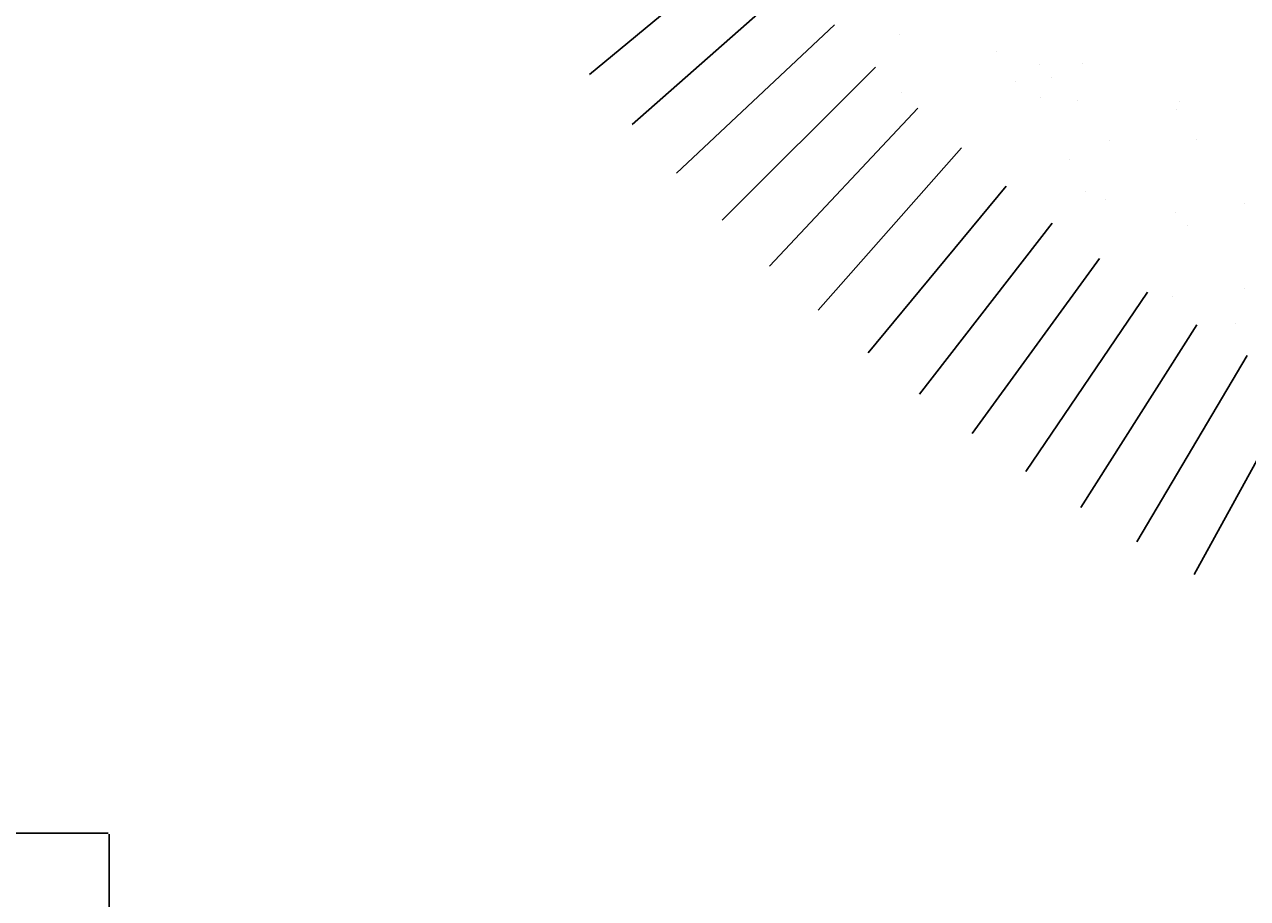
# Model space of a CAD drawing. Units: millimetres. Extents: x -857 to 54106, y -13666 to 13947.
# Tile 29 of 41: x 30856 to 31622, y 8428 to 8975. Entities that reach past the tile are written whole.
import ezdxf

# ---------------------------------------------------------------- set-up
doc = ezdxf.new("R2010")
doc.units = ezdxf.units.MM
doc.layers.add('A-ANNO-DIMS', color=2, linetype='Continuous', lineweight=18)
doc.layers.add('A-FURN', color=21, linetype='Continuous', lineweight=18)
doc.layers.add('A-HT', color=15, linetype='Continuous')
doc.styles.get("Standard").update_dxf_attribs({"font": 'arial.ttf'})
doc.dimstyles.new('ISO-25', dxfattribs={"dimtxt": 2.5, "dimasz": 2.5, "dimexe": 1.25, "dimexo": 0.625, "dimtad": 1, "dimtxsty": 'Standard', "dimcen": 2.5, "dimadec": 0, "dimazin": 0, "dimtfac": 1, "dimtmove": 0, "dimatfit": 3, "dimfxl": 1, "dimarcsym": 0})

# ---------------------------------------------------------------- blocks, each defined once
blk = doc.blocks.new('*X18')
at = {"color": 0}
for p, q in [((2.8963, 2.45263), (2.8963, 2.45263)), ((2.93684, 2.45104), (2.93684, 2.45104)), ((2.90822, 2.38569), (2.90822, 2.38569)), ((2.92931, 2.37226), (2.92931, 2.37226)), ((2.9173, 2.35563), (2.9173, 2.35563)), ((2.92651, 2.34719), (2.92651, 2.34719)), ((2.93999, 2.35469), (2.93999, 2.35469)), ((2.98305, 2.33459), (2.98305, 2.33459)), ((2.91637, 2.32581), (2.91637, 2.32581)), ((2.9424, 2.32924), (2.9424, 2.32924)), ((3.00521, 2.3239), (3.00521, 2.3239)), ((2.97001, 2.30733), (2.97001, 2.30733)), ((3.01058, 2.3101), (3.01058, 2.3101)), ((3.07819, 2.26322), (3.07819, 2.26322)), ((2.94314, 2.25835), (2.94314, 2.25835)), ((2.9486, 2.26048), (2.9486, 2.26048)), ((3.01978, 2.26172), (3.01978, 2.26172)), ((2.96969, 2.24705), (2.96969, 2.24705)), ((3.029, 2.25328), (3.029, 2.25328)), ((3.09706, 2.22014), (3.09706, 2.22014)), ((3.01373, 2.21376), (3.01373, 2.21376)), ((3.0725, 2.21342), (3.0725, 2.21342))]:
    blk.add_line(p, q, dxfattribs=at)
blk = doc.blocks.new('A$C6796526C')
at = {"layer": 'A-HT'}
for p, q in [((2.5892, 0.82372), (2.72064, 0.75146)), ((2.56896, 0.78825), (2.69808, 0.71189)), ((2.54763, 0.75343), (2.67428, 0.67305)), ((2.5252, 0.71929), (2.64927, 0.63498)), ((2.50172, 0.68588), (2.62307, 0.59771)), ((2.4772, 0.65322), (2.59572, 0.56128)), ((2.45167, 0.62135), (2.56724, 0.52574)), ((2.42514, 0.59029), (2.53766, 0.4911)), ((2.39766, 0.56009), (2.507, 0.45741)), ((2.36924, 0.53076), (2.47531, 0.4247)), ((2.33991, 0.50234), (2.44259, 0.393)), ((2.30971, 0.47486), (2.4089, 0.36234)), ((2.27865, 0.44833), (2.37427, 0.33276))]:
    blk.add_line(p, q, dxfattribs=at)
at = {"layer": 'A-HT', "extrusion": (0, 0, -1), "zscale": -1, "rotation": 180}
blk.add_blockref('*X18', (0.55, 3), dxfattribs=at)
blk = doc.blocks.new('*D47')
at = {"layer": 'A-ANNO-DIMS', "color": 0, "lineweight": -2, "transparency": 16777216}
for p, q in [((30909.25, 8468.37), (30909.25, 8061.12)), ((33620.08, 8468.37), (33620.08, 8061.12)), ((30911.75, 8062.37), (33617.58, 8062.37))]:
    blk.add_line(p, q, dxfattribs=at)
at = {"layer": 'A-ANNO-DIMS', "color": 0, "transparency": 16777216}
for points in [[(30911.75, 8062.79), (30911.75, 8061.96), (30909.25, 8062.37)], [(33617.58, 8062.79), (33617.58, 8061.96), (33620.08, 8062.37)]]:
    blk.add_solid(points, dxfattribs=at)
at = {"layer": 'Defpoints', "color": 0, "transparency": 16777216}
for p in [(30909.25, 8469), (33620.08, 8469), (33620.08, 8062.37)]:
    blk.add_point(p, dxfattribs=at)
at = {"layer": 'A-ANNO-DIMS', "color": 0, "transparency": 16777216, "insert": (32264.67, 8064.29), "char_height": 2.5, "attachment_point": 5}
blk.add_mtext('ROUND BED 2711 TYP.', dxfattribs=at)
blk = doc.blocks.new('*D48')
at = {"layer": 'A-ANNO-DIMS', "color": 0, "lineweight": -2, "transparency": 16777216}
for p, q in [((30908.63, 11089.46), (30501.38, 11089.46)), ((30502.63, 11086.96), (30502.63, 8471.5)), ((30908.63, 8469), (30501.38, 8469))]:
    blk.add_line(p, q, dxfattribs=at)
at = {"layer": 'A-ANNO-DIMS', "color": 0, "transparency": 16777216}
for points in [[(30502.21, 11086.96), (30503.05, 11086.96), (30502.63, 11089.46)], [(30502.21, 8471.5), (30503.05, 8471.5), (30502.63, 8469)]]:
    blk.add_solid(points, dxfattribs=at)
at = {"layer": 'Defpoints', "color": 0, "transparency": 16777216}
for p in [(30909.25, 11089.46), (30502.63, 8469), (30909.25, 8469)]:
    blk.add_point(p, dxfattribs=at)
at = {"layer": 'A-ANNO-DIMS', "color": 0, "transparency": 16777216, "insert": (30500.73, 9779.23), "char_height": 2.5, "attachment_point": 5, "rotation": 90}
blk.add_mtext('2620 TYP.', dxfattribs=at)

msp = doc.modelspace()

# ---------------------------------------------------------------- block references
at = {"layer": 'A-FURN', "xscale": 903.6084929786902, "yscale": 903.6084929786902, "zscale": 903.6084929786902, "rotation": 269.9999999999988}
msp.add_blockref('A$C6796526C', (30909.253, 11089.463), dxfattribs=at)

# ---------------------------------------------------------------- dimensions: what is measured, and where the dimension line sits
at = {"layer": 'A-ANNO-DIMS'}
dim = msp.add_linear_dim(base=(30502.63, 8468.999), p1=(30909.254, 11089.463), p2=(30909.254, 8468.999), angle=270, text='<> TYP.', dimstyle='ISO-25', override={"dimdec": 0, "dimrnd": 0, "dimzin": 0, "dimlunit": 2}, dxfattribs=at)
dim.commit()
dim.dimension.update_dxf_attribs({"geometry": '*D48', "text_midpoint": (30500.728, 9779.231)})
dim = msp.add_linear_dim(base=(33620.079, 8062.375), p1=(30909.254, 8468.999), p2=(33620.079, 8468.999), text='ROUND BED <> TYP.', dimstyle='ISO-25', override={"dimdec": 0, "dimrnd": 0, "dimzin": 0, "dimlunit": 2}, dxfattribs=at)
dim.commit()
dim.dimension.update_dxf_attribs({"geometry": '*D47', "text_midpoint": (32264.666, 8064.293)})

doc.saveas('drawing.dxf')
